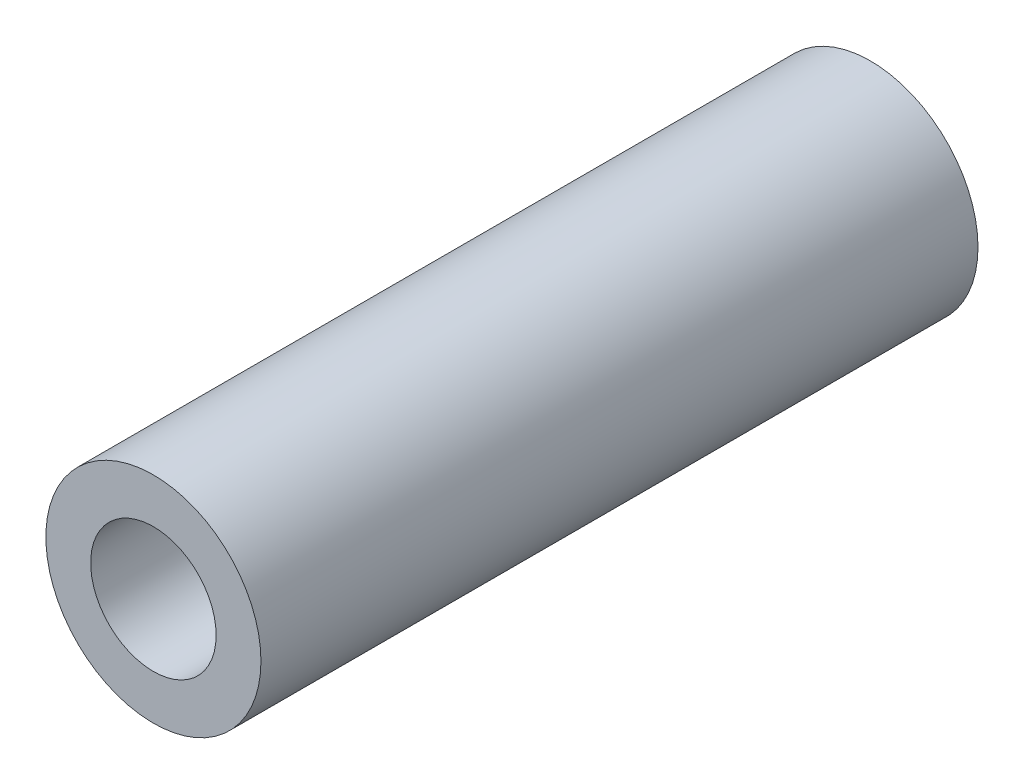
SolidWorks part; units mm, degrees
material "Plain Carbon Steel"
ref_plane "Front Plane" through (0, 0, 0) normal (0, 0, 1) x (1, 0, 0)
ref_plane "Top Plane" through (0, 0, 0) normal (0, 1, 0) x (1, 0, 0)
ref_plane "Right Plane" through (0, 0, 0) normal (1, 0, 0) x (0, 0, -1)
sketch "Bushing Profile Ø6xØ3.5" plane through (0, 0, 0) normal (0, 0, 1) x (1, 0, 0)
  circle A0 centre (0, 0) radius 3
  circle A1 centre (0, 0) radius 1.75
  dimension "D1" = 6
  dimension "D2" = 3.5
extrude "Bushing Body L20" add sketch "Bushing Profile Ø6xØ3.5" along normal mid plane 20
